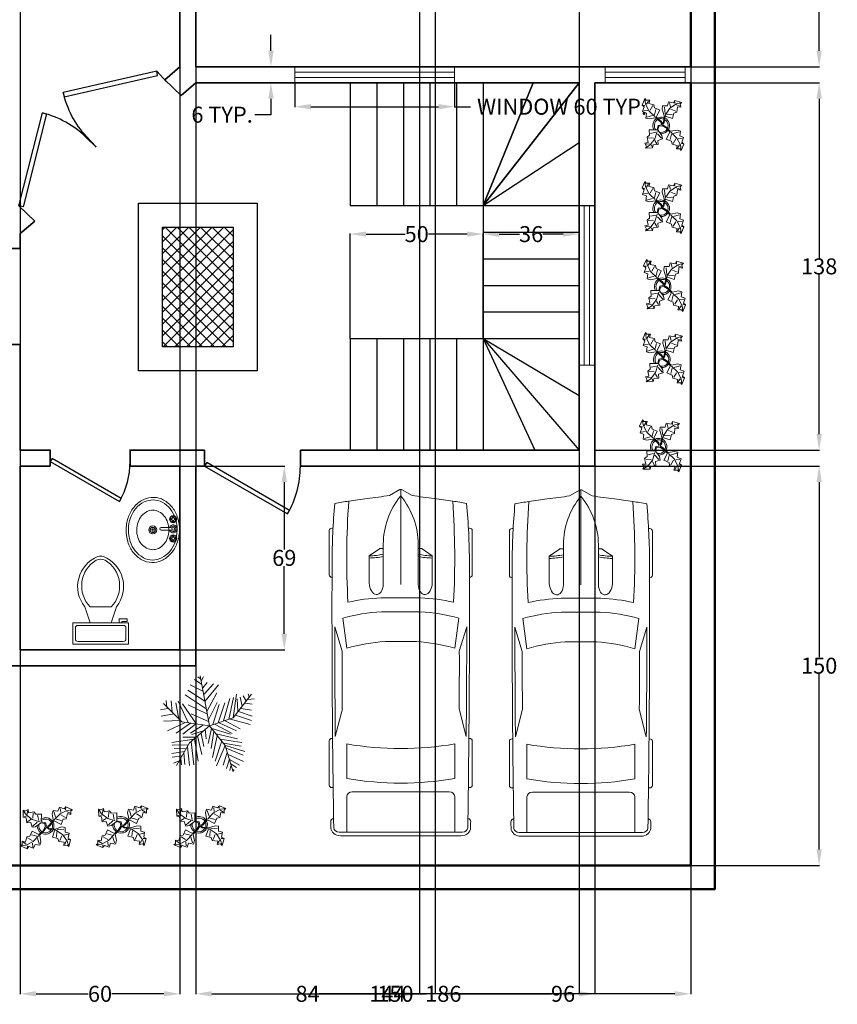
# Model space of a CAD drawing. Units: inches. Extents: x 823 to 1335, y 207 to 1074.
# Tile 2 of 6: x 1028 to 1335, y 207 to 577. Entities that reach past the tile are written whole.
import ezdxf

# ---------------------------------------------------------------- set-up
doc = ezdxf.new("R2010")
doc.units = ezdxf.units.IN
doc.header["$MEASUREMENT"] = 0
for name, color, linetype, lineweight in [('A-ANNO-DIMS', 2, 'Continuous', 18), ('A-EQPM-VEHC', 8, 'Continuous', 13), ('A-FLOR', 7, 'Continuous', 25), ('A-FLOR-PATT', 252, 'Continuous', 13), ('doors', 51, 'Continuous', 25), ('inner wall', 102, 'Continuous', 35), ('L-PLNT', 90, 'Continuous', 13), ('outer wall', 105, 'Continuous', 50), ('sanitary', 131, 'Continuous', 18), ('staircase', 10, 'Continuous', 25), ('windows', 211, 'Continuous', 18)]:
    doc.layers.add(name, color=color, linetype=linetype, lineweight=lineweight)
doc.styles.get("Standard").update_dxf_attribs({"font": 'arial.ttf'})
doc.dimstyles.get("Standard").update_dxf_attribs({"dimtxt": 6, "dimasz": 6, "dimexe": 0.18, "dimexo": 0.0625, "dimgap": 0.09, "dimtad": 0, "dimtih": 1, "dimtoh": 1, "dimdec": 0, "dimzin": 0, "dimdsep": 46, "dimlunit": 3, "dimtxsty": 'Standard', "dimcen": 0.09, "dimadec": 0, "dimazin": 0, "dimtfac": 1, "dimtdec": 0, "dimtofl": 0, "dimtmove": 0, "dimatfit": 3, "dimfxl": 1, "dimtolj": 1, "dimtzin": 0, "dimarcsym": 0})

# ---------------------------------------------------------------- blocks, each defined once
blk = doc.blocks.new('*U5')
for p, q in [((0, 0), (0, -6)), ((-40, 0), (-40, -6))]:
    blk.add_line(p, q)
blk.add_lwpolyline([(0, 0), (-34.64, 20), (-35.52, 18.48), (-0.88, -1.52)], close=True)
blk.add_arc((0, 0), 40, 150, 180)
blk = doc.blocks.new('*U4')
for p, q in [((-40, 0), (-40, 6)), ((0, 0), (0, 6))]:
    blk.add_line(p, q)
blk.add_lwpolyline([(0, 0), (-34.64, -20), (-35.52, -18.48), (-0.88, 1.52)], close=True)
blk.add_arc((0, 0), 40, 180, 210)
blk = doc.blocks.new('*U7')
for p, q in [((0, 0), (0, 6)), ((40, 0), (40, 6))]:
    blk.add_line(p, q)
blk.add_lwpolyline([(0, 0), (34.64, -20), (35.52, -18.48), (0.88, 1.52)], close=True)
blk.add_arc((0, 0), 40, 330, 360)
blk = doc.blocks.new('Toilet - top')
for p, q in [((9.5, -6), (9.5, -2)), ((-10, -8.5), (-8, -8.5)), ((-10, -9.5), (-10, -8.5)), ((-7, -9.5), (-10, -9.5)), ((-8, -8.5), (-8, -8)), ((-7, -8), (-7, -9.5)), ((-4, -8), (-6, -14)), ((4, -8), (6, -14)), ((4, -14), (-4, -14))]:
    blk.add_line(p, q)
blk.add_lwpolyline([(10.5, -8), (10.5, 0), (-10.5, 0), (-10.5, -8)], close=True)
for points in [[(-9.5, -2), (-9.5, -6)], [(8.5, -1), (-8.5, -1)], [(-8.5, -7), (8.5, -7)]]:
    blk.add_lwpolyline(points)
for centre, radius, start, end in [((-8.62, -1.88), 0.884, 81.8699, 188.1301), ((8.62, -1.88), 0.884, 351.8699, 98.1301), ((-8.62, -6.12), 0.884, 171.8699, 278.1301), ((8.62, -6.12), 0.884, 261.8699, 8.1301), ((3.52, -21.58), 12.17, 141.4691, 247.9714), ((4.2, -21.82), 11.33, 136.3677, 238.9468), ((-3.52, -21.58), 12.17, 292.0284, 38.5307), ((-4.2, -21.82), 11.33, 301.053, 43.6321), ((0, -27.88), 4, 245.7318, 294.2682), ((0, -29), 4, 254.8605, 285.1395)]:
    blk.add_arc(centre, radius, start, end)
blk = doc.blocks.new('Sink - Oval top')
for p, q in [((-1, 0), (1, 0)), ((0, 1), (0, -1))]:
    blk.add_line(p, q)
for points in [[(-12.23, 0.39, 0.117634), (-11.46, -3.36, 0.104469), (-8.88, -6.8, 0.090016), (-5.08, -9.07, 0.08192), (-0.32, -10.02, 0.08192), (4.49, -9.38, 0.090016), (8.42, -7.36, 0.104469), (11.22, -4.09, 0.117634), (12.23, -0.39, 0.117634), (11.46, 3.36, 0.104469), (8.88, 6.8, 0.090016), (5.08, 9.07, 0.08192), (0.32, 10.02, 0.08192), (-4.49, 9.38, 0.090016), (-8.42, 7.36, 0.104469), (-11.22, 4.09, 0.117634)], [(-11.29, 0.16, 0.118622), (-10.52, -3.25, 0.104678), (-8.07, -6.36, 0.089562), (-4.54, -8.37, 0.081185), (-0.13, -9.15, 0.081185), (4.3, -8.49, 0.089562), (7.89, -6.58, 0.104678), (10.42, -3.55, 0.118622), (11.29, -0.16, 0.118622), (10.52, 3.25, 0.104678), (8.07, 6.36, 0.089562), (4.54, 8.37, 0.081185), (0.13, 9.15, 0.081185), (-4.3, 8.49, 0.089562), (-7.89, 6.58, 0.104678), (-10.42, 3.55, 0.118622)], [(-7.42, 0.08, 0.118283), (-6.91, -2.17, 0.104607), (-5.29, -4.21, 0.089718), (-2.97, -5.53, 0.081436), (-0.07, -6.04, 0.081436), (2.84, -5.59, 0.089718), (5.2, -4.33, 0.104607), (6.86, -2.32, 0.118283), (7.42, -0.08, 0.118283), (6.91, 2.17, 0.104607), (5.29, 4.21, 0.089718), (2.97, 5.53, 0.081436), (0.07, 6.04, 0.081436), (-2.84, 5.59, 0.089718), (-5.2, 4.33, 0.104607), (-6.86, 2.32, 0.118283)]]:
    blk.add_lwpolyline(points, format="xyb", close=True)
for radius in [1.5, 1]:
    blk.add_circle((0, 0), radius)
blk = doc.blocks.new('Faucet - Bathroom top')
for p, q in [((-4.107, 0.125), (-4.375, 0.125)), ((-3.75, 0.4788), (-3.75, 0.75)), ((-3.5, 0.482), (-3.5, 0.75)), ((-3.1461, 0.125), (-2.875, 0.125)), ((3.143, 0.125), (2.875, 0.125)), ((3.5, 0.4788), (3.5, 0.75)), ((3.75, 0.482), (3.75, 0.75)), ((4.1039, 0.125), (4.375, 0.125)), ((-4.1039, -0.125), (-4.375, -0.125)), ((-3.75, -0.4821), (-3.75, -0.75)), ((-3.5, -0.4789), (-3.5, -0.75)), ((-3.143, -0.125), (-2.875, -0.125)), ((-0.5, -0.8639), (-0.5, -4.5)), ((0.5, -4.5), (0.5, -0.8631)), ((3.1461, -0.125), (2.875, -0.125)), ((3.5, -0.4821), (3.5, -0.75)), ((3.75, -0.4789), (3.75, -0.75)), ((4.107, -0.125), (4.375, -0.125))]:
    blk.add_line(p, q)
for centre, radius in [((-3.625, 0), 1.375), ((-4.625, 0), 0.2795), ((-3.625, 0), 0.5), ((-3.625, 1), 0.2795), ((-2.625, 0), 0.2795), ((0, 0), 0.5), ((3.625, 0), 1.375), ((2.625, 0), 0.2795), ((3.625, 0), 0.5), ((3.625, 1), 0.2795), ((4.625, 0), 0.2795), ((-3.625, -1), 0.2795), ((3.625, -1), 0.2795)]:
    blk.add_circle(centre, radius)
for centre, radius, start, end in [((-3.625, 0), 1, 105.2407, 164.2093), ((-3.625, 0), 1, 16.44125, 74.07887), ((0, 0), 1.5, 289.6514, 250.3603), ((0, 0), 1, 300.3431, 239.7554), ((3.625, 0), 1, 106.12, 164.0884), ((3.625, 0), 1, 16.23422, 73.90469), ((-3.625, 0), 1, 196.2342, 253.9047), ((-3.625, 0), 1, 286.12, 344.0884), ((3.625, 0), 1, 196.4413, 254.0789), ((3.625, 0), 1, 285.2407, 344.2093), ((0, -4.5), 0.5, 180, 0)]:
    blk.add_arc(centre, radius, start, end)
blk = doc.blocks.new('Plant - Rubber or Philodendron')
for p, q in [((-16.2005, 11.4774), (-13.9899, 8.1064)), ((-16.2005, 11.4774), (-14.8639, 10.7964)), ((-16.0159, 6.3329), (-16.2005, 11.4774)), ((-14.8639, 10.7964), (-12.6195, 11.8975)), ((-13.9899, 8.1064), (-9.5434, 4.7185)), ((-13.3174, 8.325), (-13.0735, 11.0065)), ((-12.6195, 11.8975), (-12.1909, 9.4345)), ((-12.1909, 9.4345), (-8.3829, 10.3)), ((-8.8369, 9.409), (-9.0894, 5.6095)), ((-8.3829, 10.3), (-7.0549, 8.501)), ((-7.0549, 8.501), (-3.0284, 8.6941)), ((-4.8529, 4.012), (-5.7184, 7.82)), ((-3.0284, 8.6941), (-3.0709, 3.1041)), ((4.6914, 8.8812), (5.3859, 11.2828)), ((4.6914, 8.8812), (5.5014, 4.4831)), ((5.3859, 11.2828), (8.8871, 10.7908)), ((5.9878, 10.4842), (7.1971, 6.3869)), ((10.3916, 8.7942), (6.2847, 4.4028)), ((8.8871, 10.7908), (9.9809, 13.4933)), ((9.9809, 13.4933), (13.3837, 12.301)), ((15.3859, 11.3055), (10.3916, 8.7942)), ((10.5828, 12.6946), (10.8893, 9.7953)), ((14.2977, 6.1031), (10.9934, 7.9956)), ((13.3837, 12.301), (14.68, 13.9039)), ((14.5816, 13.2037), (14.3848, 11.8033)), ((14.68, 13.9039), (19.3848, 11.8146)), ((15.7909, 9.1065), (14.8995, 5.3044)), ((15.2875, 10.6053), (17.5907, 9.2105)), ((19.3848, 11.8146), (15.3859, 11.3055)), ((18.1925, 8.4119), (15.7909, 9.1065)), ((19.3848, 11.8146), (18.1868, 10.9119)), ((18.1868, 10.9119), (18.1925, 8.4119)), ((-14.0069, 5.8704), (-16.0159, 6.3329)), ((-15.3434, 6.5514), (-13.9984, 6.9884)), ((-13.5868, 2.2894), (-14.0069, 5.8704)), ((-10.6784, 2.491), (-13.5868, 2.2894)), ((-13.1329, 3.1804), (-10.6614, 4.727)), ((-9.5858, -0.8715), (-10.6784, 2.491)), ((-9.5434, 4.7185), (-4.1917, 2.9888)), ((-9.1318, 0.0195), (-5.9793, 2.9025)), ((-7.1228, -0.443), (-3.5248, 2.2131)), ((-3.5248, 2.2131), (-3.3011, 2.4355)), ((-3.3011, 2.4355), (-0.5306, 1.7947)), ((-3.0709, 3.1041), (0.0797, 2.3163)), ((-0.5306, 1.7947), (-0.2255, -0.5527)), ((-0.5306, 1.7947), (-0.5306, 1.7947)), ((0.0797, 2.3163), (0.4866, -0.031)), ((0.4866, -0.031), (2.1141, 0.2298)), ((2.1141, 0.2298), (5.4346, 3.9146)), ((6.1032, 3.6844), (2.8262, -0.031)), ((5.4346, 3.9146), (5.5014, 4.4831)), ((11.1089, 1.1958), (6.1032, 3.6844)), ((7.7005, 4.8881), (11.5025, 3.9967)), ((12.7005, 4.8994), (11.1089, 1.1958)), ((14.8995, 5.3044), (12.7005, 4.8994)), ((-11.3237, -7.2629), (-9.7321, -3.5593)), ((-6.3237, -7.2516), (-10.1257, -6.3602)), ((-9.7321, -3.5593), (-4.7264, -6.0479)), ((-7.1228, -0.443), (-9.5858, -0.8715)), ((-9.0148, -11.1577), (-4.9047, -6.8122)), ((-2.019, -3.6148), (-4.7264, -6.0479)), ((-4.1246, -6.8466), (-4.0579, -6.2781)), ((-3.3146, -11.2447), (-4.1246, -6.8466)), ((-4.0579, -6.2781), (-0.9375, -3.1608)), ((-2.019, -3.6148), (-0.2255, -0.5527)), ((-0.9375, -3.1608), (0.5883, -0.8135)), ((0.5883, -0.8135), (2.2447, -2.0916)), ((2.8262, -0.031), (1.3003, -0.5527)), ((1.3003, -0.5527), (2.4193, -1.4655)), ((2.2447, -2.0916), (6.7108, -2.6626)), ((2.4193, -1.4655), (6.895, -2.1175)), ((4.943, -7.9659), (6.7108, -2.6626)), ((11.6605, -0.5413), (6.895, -2.1175)), ((12.3677, -6.1981), (7.219, -2.6772)), ((8.125, -4.0768), (7.7715, -7.9659)), ((8.3544, -2.7453), (13.1973, -2.1704)), ((10.2463, -10.4408), (11.6605, -6.9053)), ((11.6605, -0.5413), (14.1354, -0.8948)), ((15.5496, -10.7943), (12.3677, -6.1981)), ((16.2567, -5.8446), (13.4283, -6.5517)), ((14.1354, -0.8948), (14.1354, -4.4304)), ((14.1354, -4.4304), (16.9638, -5.1375)), ((16.9638, -5.1375), (16.2567, -8.673)), ((-18.008, -14.1781), (-16.8101, -13.2754)), ((-18.008, -14.1781), (-14.0091, -13.669)), ((-16.8157, -10.7754), (-14.4141, -11.4699)), ((-16.8101, -13.2754), (-16.8157, -10.7754)), ((-13.9107, -12.9688), (-16.2139, -11.574)), ((-14.4141, -11.4699), (-13.5228, -7.6679)), ((-14.0091, -13.669), (-9.0148, -11.1577)), ((-13.5228, -7.6679), (-11.3237, -7.2629)), ((-12.921, -8.4665), (-9.6166, -10.359)), ((-9.206, -15.0581), (-9.5126, -12.1588)), ((-7.5103, -13.1543), (-8.6042, -15.8568)), ((-4.0092, -13.6463), (-7.5103, -13.1543)), ((-4.611, -12.8477), (-5.8203, -8.7504)), ((-3.3146, -11.2447), (-4.0092, -13.6463)), ((8.8321, -9.0266), (4.943, -7.9659)), ((9.5392, -11.1479), (8.8321, -9.0266)), ((13.4283, -11.5015), (9.5392, -11.1479)), ((13.0748, -13.9763), (13.4283, -11.5015)), ((15.5496, -13.6228), (13.0748, -13.9763)), ((14.8425, -10.7943), (13.7819, -13.2692)), ((16.6103, -14.6834), (15.5496, -10.7943)), ((16.6103, -14.6834), (15.5496, -13.6228)), ((17.3174, -9.7337), (15.9032, -9.7337)), ((16.2567, -8.673), (18.0245, -9.7337)), ((18.0245, -9.7337), (16.6103, -14.6834)), ((-13.3032, -16.2674), (-18.008, -14.1781)), ((-12.0069, -14.6645), (-13.3032, -16.2674)), ((-13.2048, -15.5672), (-13.008, -14.1668)), ((-8.6042, -15.8568), (-12.0069, -14.6645))]:
    blk.add_line(p, q)
for centre, radius, start, end in [((0.0308, 0.1664), 6, 178.6147, 235.1169), ((0.0308, 0.1664), 5, 168.1647, 238.6725), ((0, 0), 6.1275, 34.37569, 120.1028), ((-0.0601, -0.2075), 5.2461, 33.82192, 124.9414), ((-0.2664, 0.1682), 5.2775, 338.4094, 20.03007), ((-0.098, 0.1364), 6.1288, 341.2017, 26.09184), ((-0.0234, 0.3825), 6.1492, 242.5812, 331.2714), ((-0.1102, 0.4886), 5.2883, 247.3711, 327.472)]:
    blk.add_arc(centre, radius, start, end)
blk = doc.blocks.new('*U18')
for p, q in [((46.55, 38.89), (22.35, 38.89)), ((136.7, 38.89), (160.9, 38.89)), ((21.1, 37.41), (21.1, 36.83)), ((47.8, 37.39), (47.8, 37.41)), ((87.99, 31.87), (74.76, 35.92)), ((134.31, 35.6), (119.29, 31.78)), ((135.45, 37.07), (135.45, 37.41)), ((162.15, 37.41), (162.15, 36.77)), ((186.47, -33.5), (186.47, 33.5)), ((188.4, -32.76), (188.4, 32.76)), ((70.03, 31.54), (86.41, 29.35)), ((138.42, 29.35), (157.25, 29.35)), ((186.47, 29.35), (167.01, 29.35)), ((164.52, 26.39), (164.52, -26.39)), ((32.27, 11.63), (36.13, 17.17)), ((36.13, 17.17), (50.94, 17.17)), ((32.12, 9.51), (32.12, 11.15)), ((58.92, -10.77), (58.92, 10.77)), ((3.27, 6.13), (0.1, 0.41)), ((29.77, 9.51), (51.68, 9.51)), ((66.55, -10.53), (66.55, 10.53)), ((82.74, 8.5), (82.74, -8.5)), ((186.47, -10.53), (186.47, 10.53)), ((0, 0), (51.68, 0)), ((0.1, -0.41), (3.27, -6.13)), ((29.77, -9.51), (51.68, -9.51)), ((32.12, -9.51), (32.12, -11.15)), ((32.27, -11.63), (36.13, -17.17)), ((36.13, -17.17), (50.94, -17.17)), ((86.41, -29.35), (70.03, -31.54)), ((87.99, -31.87), (74.76, -35.92)), ((134.31, -35.6), (119.29, -31.78)), ((157.25, -29.35), (138.42, -29.35)), ((167.01, -29.35), (186.47, -29.35)), ((21.1, -37.41), (21.1, -36.83)), ((47.8, -37.39), (47.8, -37.41)), ((135.45, -37.07), (135.45, -37.41)), ((162.15, -37.41), (162.15, -36.77)), ((46.55, -38.89), (22.35, -38.89)), ((136.7, -38.89), (160.9, -38.89))]:
    blk.add_line(p, q)
for centre, major_axis, ratio, start_param, end_param in [((22.35, 37.41), (0, -1.48), 0.842304, 3.141593, 4.712389), ((64.48, -10555.62), (0, 10593.03), 0.842304, -0.013397, 0.002797), ((46.55, 37.41), (0, 1.48), 0.842304, -1.570796, 0), ((136.7, 37.41), (0, -1.48), 0.842304, 3.141593, 4.712389), ((160.9, 37.41), (0, 1.48), 0.842304, -1.570796, 0), ((180.63, 35.84), (0, 2.22), 0.842304, -0.013017, 1.249894), ((64.48, -10556.36), (0, 10595.31), 0.842304, -0.013397, -0.013017), ((183.98, 32.76), (0, -5.25), 0.842304, 1.570796, 3.128196), ((266.03, -27.52), (0, 313.31), 0.842304, 1.367076, 1.39176), ((41.19, -490.86), (0, 528.23), 0.842304, 0.00281, 0.075598), ((64.48, -10555.62), (0, -10591.55), 0.842304, 3.133765, 3.140441), ((183.98, 33.5), (0, -2.96), 0.842304, 1.570796, 3.128196), ((259.18, -27.52), (0, -305.3), 0.842304, 4.528606, 4.561838), ((37.47, -593.96), (0, -623.33), 0.842304, 3.096046, 3.200911), ((134.4, 5.39), (0, -89.78), 0.842304, 4.449482, 4.652344), ((135.29, 5.39), (0, 81.77), 0.842304, 1.245306, 1.50788), ((149.6, 2.8), (0, -79.58), 0.842304, 4.372215, 4.640744), ((95.79, -3666.35), (0, -3698.24), 0.842304, 3.134049, 3.144098), ((17.08, 0), (0, 147.02), 0.842304, 4.511394, 4.913384), ((35.91, 0), (0, 147.02), 0.842304, 4.511394, 4.913384), ((167.01, 26.39), (0, 2.96), 0.842304, 0, 1.570796), ((-204.49, 52.4), (0, -250.96), 0.842304, 1.385369, 1.434372), ((13.04, 17.01), (0, 27.42), 0.842304, 4.435146, 4.718221), ((14.2, 17.01), (0, 27.42), 0.842304, 4.435146, 4.718221), ((50.79, 13.34), (6.34, -0.36), 0.603834, -1.395552, 1.581315), ((32.75, 11.15), (0, 0.74), 0.842304, 0.879714, 1.570796), ((29.77, -46.66), (0, 56.17), 0.842304, 0, 0.590319), ((0.62, 0), (0, -0.74), 0.842304, 4.131459, 5.293319), ((29.77, 46.66), (0, 56.17), 0.842304, 2.551274, 3.141593), ((-204.49, -52.4), (0, 250.96), 0.842304, -1.434372, -1.385369), ((13.04, -17.01), (0, -27.42), 0.842304, 1.564964, 1.848039), ((14.2, -17.01), (0, -27.42), 0.842304, 1.564964, 1.848039), ((135.29, -5.39), (0, -81.77), 0.842304, -1.50788, -1.245306), ((149.6, -2.8), (0, -79.58), 0.842304, -1.499151, -1.230623), ((32.75, -11.15), (0, -0.74), 0.842304, 4.712389, 5.403472), ((134.4, -5.39), (0, -89.78), 0.842304, -1.510751, -1.307889), ((259.18, 27.52), (0, 305.3), 0.842304, 1.721348, 1.754579), ((167.01, -26.39), (0, -2.96), 0.842304, 4.712389, 6.283185), ((266.03, 27.52), (0, 313.31), 0.842304, 1.749832, 1.774517), ((37.47, 593.96), (0, -623.33), 0.842304, -0.059319, 0.045547), ((95.79, 3666.35), (0, -3698.24), 0.842304, -0.002505, 0.007544), ((41.19, 490.86), (0, -528.23), 0.842304, -0.075598, -0.00281), ((22.35, -37.41), (0, 1.48), 0.842304, 1.570796, 3.141593), ((64.48, 10555.62), (0, 10593.03), 0.842304, 3.138796, 3.15499), ((46.55, -37.41), (0, -1.48), 0.842304, 0, 1.570796), ((64.48, 10555.62), (0, -10591.55), 0.842304, 0.001152, 0.007828), ((136.7, -37.41), (0, -1.48), 0.842304, -1.570796, 0), ((160.9, -37.41), (0, 1.48), 0.842304, 3.141593, 4.712389), ((180.63, -35.84), (0, -2.22), 0.842304, -1.249894, 0.013017), ((183.98, -33.5), (0, 2.96), 0.842304, 3.15499, 4.712389), ((183.98, -32.76), (0, -5.25), 0.842304, 0.013397, 1.570796), ((64.48, 10556.36), (0, 10595.31), 0.842304, 3.15461, 3.15499)]:
    blk.add_ellipse(centre, major_axis=major_axis, ratio=ratio, start_param=start_param, end_param=end_param)
at = {"extrusion": (0, 0, -1)}
blk.add_ellipse((50.79, -13.34), major_axis=(6.34, 0.36), ratio=0.603834, start_param=-1.395552, end_param=1.581315, dxfattribs=at)
blk = doc.blocks.new('*U20')
for p, q in [((0, 0), (-10.5, 57)), ((-7.288, 39.707), (-21.778, 46.673)), ((-8.737, 47.138), (-17.069, 52.711)), ((-10.186, 53.64), (-13.084, 55.962)), ((-9.099, 51.782), (-6.563, 55.962)), ((-7.65, 43.423), (-2.578, 49.46)), ((-5.839, 35.992), (4.667, 48.067)), ((-5.114, 27.632), (10.463, 46.673)), ((-3.665, 19.273), (-27.574, 35.527)), ((-5.114, 28.097), (-24.676, 40.636)), ((-2.941, 16.486), (8.652, 37.85)), ((27, 9), (48, 36)), ((27.127, 9.056), (31.112, 35.992)), ((38.719, 34.134), (41.979, 28.561)), ((44.153, 36.456), (45.239, 32.741)), ((-31.5, 4.5), (-52.5, 25.5)), ((-48.585, 21.131), (-49.309, 29.026)), ((-43.513, 28.561), (-42.427, 15.558)), ((-38.442, 26.239), (-34.819, 7.663)), ((-35.544, 28.097), (-24.314, 3.947)), ((-14.533, 2.09), (-30.834, 25.31)), ((-24.314, 23.917), (-2.941, 13.7)), ((-1.129, 6.734), (9.014, 26.704)), ((3.942, 1.625), (11.187, 24.381)), ((10.101, 3.483), (17.708, 26.239)), ((16.259, 5.805), (23.142, 31.348)), ((22.055, 7.198), (27.489, 32.277)), ((31.836, 30.883), (32.561, 16.486)), ((35.096, 32.741), (37.27, 22.524)), ((40.53, 25.775), (48.862, 24.846)), ((43.791, 29.954), (51.036, 30.883)), ((-47.498, 19.737), (-55.83, 18.344)), ((-40.615, 13.7), (-55.105, 10.913)), ((-20.691, 13.7), (-1.129, 4.876)), ((29.662, 12.307), (48.137, 6.269)), ((33.285, 16.486), (48.862, 10.913)), ((36.183, 19.737), (48.137, 17.88)), ((-33.37, 6.269), (-52.207, 5.34)), ((-28.299, 3.483), (-47.86, -5.805)), ((-21.416, 3.018), (-38.079, -8.128)), ((0, 0), (-31.5, 4.5)), ((-15.982, 2.09), (-30.11, -9.521)), ((0, 0), (-22.5, -19.5)), ((-6.563, 1.161), (-21.416, -8.128)), ((0, 0), (27, 9)), ((0, 0), (18, -22.5)), ((6.478, 1.625), (26.04, -8.592)), ((11.187, 3.483), (30.749, -5.805)), ((18.07, 5.805), (35.096, -3.483)), ((24.229, 7.663), (46.688, 1.625)), ((-6.563, -5.805), (-19.967, -9.985)), ((-9.461, -8.592), (-6.201, -23.453)), ((-4.752, -3.483), (-3.665, -14.629)), ((2.493, -3.019), (-1.491, -20.202)), ((1.769, -2.555), (24.229, -9.521)), ((5.029, -6.27), (2.131, -25.775)), ((7.565, -9.056), (32.198, -14.629)), ((-17.431, -15.094), (-42.789, -18.809)), ((-24.314, -21.596), (-42.427, -22.06)), ((-22.5, -19.5), (-37.5, -45)), ((-15.257, -12.772), (-30.11, -12.772)), ((-20.691, -18.345), (-17.793, -44.352)), ((-17.069, -15.094), (-12.721, -40.172)), ((-13.446, -11.378), (-8.737, -32.741)), ((9.014, -11.378), (3.58, -35.992)), ((14.085, -16.951), (6.478, -40.172)), ((12.274, -15.094), (36.907, -18.809)), ((16.259, -19.738), (36.183, -22.989)), ((-28.299, -29.026), (-42.789, -31.348)), ((-26.849, -26.24), (-40.253, -25.775)), ((-29.023, -30.884), (-27.936, -43.887)), ((-25.038, -23.918), (-22.865, -45.281)), ((18.07, -22.524), (8.289, -45.745)), ((20.244, -30.419), (15.897, -44.816)), ((18, -22.5), (27, -52.5)), ((18.433, -22.524), (40.53, -29.026)), ((19.157, -25.311), (38.719, -33.206)), ((21.331, -32.741), (39.081, -40.636)), ((-30.834, -34.135), (-42.427, -35.528)), ((-34.457, -39.708), (-40.978, -42.494)), ((-32.646, -36.921), (-31.921, -44.352)), ((22.78, -37.85), (19.519, -48.532)), ((22.78, -38.314), (34.372, -44.816)), ((24.591, -43.423), (30.749, -47.603)), ((24.591, -45.745), (23.142, -50.854)), ((26.764, -49.925), (28.213, -50.854))]:
    blk.add_line(p, q)
blk = doc.blocks.new('WIN-60IN')
for p, q in [((0, 0), (0, 60)), ((0, 60), (6, 60)), ((2, 0), (2, 60)), ((4, 60), (4, 0)), ((6, 60), (6, 0)), ((6, 0), (0, 0))]:
    blk.add_line(p, q)
blk = doc.blocks.new('WIN-30IN')
for p, q in [((0, 6), (30, 6)), ((0, 0), (0, 6)), ((0, 4), (30, 4)), ((30, 6), (30, 0)), ((30, 2), (0, 2)), ((30, 0), (0, 0))]:
    blk.add_line(p, q)
blk = doc.blocks.new('*D46')
at = {"layer": 'A-ANNO-DIMS', "color": 0, "lineweight": -2, "transparency": 16777216}
for p, q in [((1131.5, 553.54), (1131.5, 544.43)), ((1191.5, 553.54), (1191.5, 544.43)), ((1137.5, 544.61), (1185.5, 544.61)), ((1191.5, 544.61), (1197.5, 544.61))]:
    blk.add_line(p, q, dxfattribs=at)
for points in [[(1137.5, 545.61), (1137.5, 543.61), (1131.5, 544.61)], [(1185.5, 545.61), (1185.5, 543.61), (1191.5, 544.61)]]:
    blk.add_solid(points, dxfattribs=at)
at = {"layer": 'Defpoints', "color": 0, "lineweight": -2, "transparency": 16777216}
for p in [(1131.5, 553.61), (1191.5, 553.61), (1191.5, 544.61)]:
    blk.add_point(p, dxfattribs=at)
at = {"layer": 'A-ANNO-DIMS', "color": 0, "transparency": 16777216, "insert": (1231.87, 544.61), "char_height": 6, "attachment_point": 5}
blk.add_mtext('\\A1;WINDOW 60 TYP.', dxfattribs=at)
blk = doc.blocks.new('*D47')
at = {"layer": 'A-ANNO-DIMS', "color": 0, "lineweight": -2, "transparency": 16777216}
for p, q in [((1122.5, 565.61), (1122.5, 571.61)), ((1131.44, 559.61), (1122.32, 559.61)), ((1131.44, 553.61), (1122.32, 553.61)), ((1122.5, 547.61), (1122.5, 541.61)), ((1122.5, 541.61), (1116.5, 541.61))]:
    blk.add_line(p, q, dxfattribs=at)
for points in [[(1121.5, 565.61), (1123.5, 565.61), (1122.5, 559.61)], [(1121.5, 547.61), (1123.5, 547.61), (1122.5, 553.61)]]:
    blk.add_solid(points, dxfattribs=at)
at = {"layer": 'Defpoints', "color": 0, "lineweight": -2, "transparency": 16777216}
for p in [(1131.5, 559.61), (1122.5, 553.61), (1131.5, 553.61)]:
    blk.add_point(p, dxfattribs=at)
at = {"layer": 'A-ANNO-DIMS', "color": 0, "transparency": 16777216, "insert": (1104.13, 541.61), "char_height": 6, "attachment_point": 5}
blk.add_mtext('\\A1;6 TYP.', dxfattribs=at)
blk = doc.blocks.new('*D61')
at = {"layer": 'A-ANNO-DIMS', "color": 0, "lineweight": -2, "transparency": 16777216}
for p, q in [((1028.26, 847.54), (1028.26, 211.18)), ((1088.26, 847.54), (1088.26, 211.18)), ((1034.26, 211.36), (1053.87, 211.36)), ((1082.26, 211.36), (1062.66, 211.36))]:
    blk.add_line(p, q, dxfattribs=at)
for points in [[(1034.26, 212.36), (1034.26, 210.36), (1028.26, 211.36)], [(1082.26, 212.36), (1082.26, 210.36), (1088.26, 211.36)]]:
    blk.add_solid(points, dxfattribs=at)
at = {"layer": 'Defpoints', "color": 0, "lineweight": -2, "transparency": 16777216}
for p in [(1028.26, 847.61), (1088.26, 847.61), (1088.26, 211.36)]:
    blk.add_point(p, dxfattribs=at)
at = {"layer": 'A-ANNO-DIMS', "color": 0, "transparency": 16777216, "insert": (1058.26, 211.36), "char_height": 6, "attachment_point": 5}
blk.add_mtext('\\A1;60', dxfattribs=at)
blk = doc.blocks.new('*D62')
at = {"layer": 'A-ANNO-DIMS', "color": 0, "lineweight": -2, "transparency": 16777216}
for p, q in [((1094.26, 775.54), (1094.26, 211.18)), ((1238.26, 775.54), (1238.26, 211.18)), ((1100.26, 211.36), (1159.84, 211.36)), ((1232.26, 211.36), (1172.69, 211.36))]:
    blk.add_line(p, q, dxfattribs=at)
for points in [[(1100.26, 212.36), (1100.26, 210.36), (1094.26, 211.36)], [(1232.26, 212.36), (1232.26, 210.36), (1238.26, 211.36)]]:
    blk.add_solid(points, dxfattribs=at)
at = {"layer": 'Defpoints', "color": 0, "lineweight": -2, "transparency": 16777216}
for p in [(1094.26, 775.61), (1238.26, 775.61), (1238.26, 211.36)]:
    blk.add_point(p, dxfattribs=at)
at = {"layer": 'A-ANNO-DIMS', "color": 0, "transparency": 16777216, "insert": (1166.26, 211.36), "char_height": 6, "attachment_point": 5}
blk.add_mtext('\\A1;144', dxfattribs=at)
blk = doc.blocks.new('*D68')
at = {"layer": 'A-ANNO-DIMS', "color": 0, "lineweight": -2, "transparency": 16777216}
for p, q in [((1094.26, 709.54), (1094.26, 211.18)), ((1178.26, 709.54), (1178.26, 211.18)), ((1100.26, 211.36), (1131.88, 211.36)), ((1172.26, 211.36), (1140.64, 211.36))]:
    blk.add_line(p, q, dxfattribs=at)
for points in [[(1100.26, 212.36), (1100.26, 210.36), (1094.26, 211.36)], [(1172.26, 212.36), (1172.26, 210.36), (1178.26, 211.36)]]:
    blk.add_solid(points, dxfattribs=at)
at = {"layer": 'Defpoints', "color": 0, "lineweight": -2, "transparency": 16777216}
for p in [(1094.26, 709.61), (1178.26, 709.61), (1178.26, 211.36)]:
    blk.add_point(p, dxfattribs=at)
at = {"layer": 'A-ANNO-DIMS', "color": 0, "transparency": 16777216, "insert": (1136.26, 211.36), "char_height": 6, "attachment_point": 5}
blk.add_mtext('\\A1;84', dxfattribs=at)
blk = doc.blocks.new('*D69')
at = {"layer": 'A-ANNO-DIMS', "color": 0, "lineweight": -2, "transparency": 16777216}
for p, q in [((1184.26, 709.54), (1184.26, 211.18)), ((1280.26, 709.54), (1280.26, 211.18)), ((1190.26, 211.36), (1227.88, 211.36)), ((1274.26, 211.36), (1236.65, 211.36))]:
    blk.add_line(p, q, dxfattribs=at)
for points in [[(1190.26, 212.36), (1190.26, 210.36), (1184.26, 211.36)], [(1274.26, 212.36), (1274.26, 210.36), (1280.26, 211.36)]]:
    blk.add_solid(points, dxfattribs=at)
at = {"layer": 'Defpoints', "color": 0, "lineweight": -2, "transparency": 16777216}
for p in [(1184.26, 709.61), (1280.26, 709.61), (1280.26, 211.36)]:
    blk.add_point(p, dxfattribs=at)
at = {"layer": 'A-ANNO-DIMS', "color": 0, "transparency": 16777216, "insert": (1232.26, 211.36), "char_height": 6, "attachment_point": 5}
blk.add_mtext('\\A1;96', dxfattribs=at)
blk = doc.blocks.new('*D71')
at = {"layer": 'A-ANNO-DIMS', "color": 0, "lineweight": -2, "transparency": 16777216}
for p, q in [((1094.26, 559.54), (1094.26, 211.18)), ((1280.26, 559.54), (1280.26, 211.18)), ((1100.26, 211.36), (1180.83, 211.36)), ((1274.26, 211.36), (1193.7, 211.36))]:
    blk.add_line(p, q, dxfattribs=at)
for points in [[(1100.26, 212.36), (1100.26, 210.36), (1094.26, 211.36)], [(1274.26, 212.36), (1274.26, 210.36), (1280.26, 211.36)]]:
    blk.add_solid(points, dxfattribs=at)
at = {"layer": 'Defpoints', "color": 0, "lineweight": -2, "transparency": 16777216}
for p in [(1094.26, 559.61), (1280.26, 559.61), (1280.26, 211.36)]:
    blk.add_point(p, dxfattribs=at)
at = {"layer": 'A-ANNO-DIMS', "color": 0, "transparency": 16777216, "insert": (1187.26, 211.36), "char_height": 6, "attachment_point": 5}
blk.add_mtext('\\A1;186', dxfattribs=at)
blk = doc.blocks.new('*D72')
at = {"layer": 'A-ANNO-DIMS', "color": 0, "lineweight": -2, "transparency": 16777216}
for p, q in [((1280.32, 703.61), (1328.69, 703.61)), ((1328.51, 697.61), (1328.51, 634.71)), ((1328.51, 565.61), (1328.51, 628.5)), ((1280.32, 559.61), (1328.69, 559.61))]:
    blk.add_line(p, q, dxfattribs=at)
for points in [[(1327.51, 697.61), (1329.51, 697.61), (1328.51, 703.61)], [(1327.51, 565.61), (1329.51, 565.61), (1328.51, 559.61)]]:
    blk.add_solid(points, dxfattribs=at)
at = {"layer": 'Defpoints', "color": 0, "lineweight": -2, "transparency": 16777216}
for p in [(1280.26, 703.61), (1328.51, 703.61), (1280.26, 559.61)]:
    blk.add_point(p, dxfattribs=at)
at = {"layer": 'A-ANNO-DIMS', "color": 0, "transparency": 16777216, "insert": (1328.51, 631.61), "char_height": 6, "attachment_point": 5}
blk.add_mtext('\\A1;144', dxfattribs=at)
blk = doc.blocks.new('*D75')
at = {"layer": 'A-ANNO-DIMS', "color": 0, "lineweight": -2, "transparency": 16777216}
for p, q in [((1028.26, 340.54), (1028.26, 211.18)), ((1088.26, 340.54), (1088.26, 211.18)), ((1034.26, 211.36), (1053.87, 211.36)), ((1082.26, 211.36), (1062.66, 211.36))]:
    blk.add_line(p, q, dxfattribs=at)
for points in [[(1034.26, 212.36), (1034.26, 210.36), (1028.26, 211.36)], [(1082.26, 212.36), (1082.26, 210.36), (1088.26, 211.36)]]:
    blk.add_solid(points, dxfattribs=at)
at = {"layer": 'Defpoints', "color": 0, "lineweight": -2, "transparency": 16777216}
for p in [(1028.26, 340.61), (1088.26, 340.61), (1088.26, 211.36)]:
    blk.add_point(p, dxfattribs=at)
at = {"layer": 'A-ANNO-DIMS', "color": 0, "transparency": 16777216, "insert": (1058.26, 211.36), "char_height": 6, "attachment_point": 5}
blk.add_mtext('\\A1;60', dxfattribs=at)
blk = doc.blocks.new('*D76')
at = {"layer": 'A-ANNO-DIMS', "color": 0, "lineweight": -2, "transparency": 16777216}
for p, q in [((1088.32, 409.61), (1127.69, 409.61)), ((1127.51, 403.61), (1127.51, 378.26)), ((1127.51, 346.61), (1127.51, 371.95)), ((1088.32, 340.61), (1127.69, 340.61))]:
    blk.add_line(p, q, dxfattribs=at)
for points in [[(1126.51, 403.61), (1128.51, 403.61), (1127.51, 409.61)], [(1126.51, 346.61), (1128.51, 346.61), (1127.51, 340.61)]]:
    blk.add_solid(points, dxfattribs=at)
at = {"layer": 'Defpoints', "color": 0, "lineweight": -2, "transparency": 16777216}
for p in [(1088.26, 409.61), (1088.26, 340.61), (1127.51, 340.61)]:
    blk.add_point(p, dxfattribs=at)
at = {"layer": 'A-ANNO-DIMS', "color": 0, "transparency": 16777216, "insert": (1127.51, 375.11), "char_height": 6, "attachment_point": 5}
blk.add_mtext('\\A1;69', dxfattribs=at)
blk = doc.blocks.new('*D77')
at = {"layer": 'A-ANNO-DIMS', "color": 0, "lineweight": -2, "transparency": 16777216}
for p, q in [((1094.26, 409.54), (1094.26, 211.18)), ((1244.26, 409.54), (1244.26, 211.18)), ((1100.26, 211.36), (1162.84, 211.36)), ((1238.26, 211.36), (1175.69, 211.36))]:
    blk.add_line(p, q, dxfattribs=at)
for points in [[(1100.26, 212.36), (1100.26, 210.36), (1094.26, 211.36)], [(1238.26, 212.36), (1238.26, 210.36), (1244.26, 211.36)]]:
    blk.add_solid(points, dxfattribs=at)
at = {"layer": 'Defpoints', "color": 0, "lineweight": -2, "transparency": 16777216}
for p in [(1094.26, 409.61), (1244.26, 409.61), (1244.26, 211.36)]:
    blk.add_point(p, dxfattribs=at)
at = {"layer": 'A-ANNO-DIMS', "color": 0, "transparency": 16777216, "insert": (1169.26, 211.36), "char_height": 6, "attachment_point": 5}
blk.add_mtext('\\A1;150', dxfattribs=at)
blk = doc.blocks.new('*D78')
at = {"layer": 'A-ANNO-DIMS', "color": 0, "lineweight": -2, "transparency": 16777216}
for p, q in [((1244.32, 553.61), (1328.69, 553.61)), ((1328.51, 547.61), (1328.51, 487.76)), ((1328.51, 421.61), (1328.51, 481.45)), ((1244.32, 415.61), (1328.69, 415.61))]:
    blk.add_line(p, q, dxfattribs=at)
for points in [[(1327.51, 547.61), (1329.51, 547.61), (1328.51, 553.61)], [(1327.51, 421.61), (1329.51, 421.61), (1328.51, 415.61)]]:
    blk.add_solid(points, dxfattribs=at)
at = {"layer": 'Defpoints', "color": 0, "lineweight": -2, "transparency": 16777216}
for p in [(1244.26, 553.61), (1328.51, 553.61), (1244.26, 415.61)]:
    blk.add_point(p, dxfattribs=at)
at = {"layer": 'A-ANNO-DIMS', "color": 0, "transparency": 16777216, "insert": (1328.51, 484.61), "char_height": 6, "attachment_point": 5}
blk.add_mtext('\\A1;138', dxfattribs=at)
blk = doc.blocks.new('*D79')
at = {"layer": 'A-ANNO-DIMS', "color": 0, "lineweight": -2, "transparency": 16777216}
for p, q in [((1244.32, 409.61), (1328.69, 409.61)), ((1328.51, 403.61), (1328.51, 337.76)), ((1328.51, 265.61), (1328.51, 331.45)), ((1280.32, 259.61), (1328.69, 259.61))]:
    blk.add_line(p, q, dxfattribs=at)
for points in [[(1327.51, 403.61), (1329.51, 403.61), (1328.51, 409.61)], [(1327.51, 265.61), (1329.51, 265.61), (1328.51, 259.61)]]:
    blk.add_solid(points, dxfattribs=at)
at = {"layer": 'Defpoints', "color": 0, "lineweight": -2, "transparency": 16777216}
for p in [(1244.26, 409.61), (1328.51, 409.61), (1280.26, 259.61)]:
    blk.add_point(p, dxfattribs=at)
at = {"layer": 'A-ANNO-DIMS', "color": 0, "transparency": 16777216, "insert": (1328.51, 334.61), "char_height": 6, "attachment_point": 5}
blk.add_mtext('\\A1;150', dxfattribs=at)
blk = doc.blocks.new('*D80')
at = {"layer": 'A-ANNO-DIMS', "color": 0, "lineweight": -2, "transparency": 16777216}
for p, q in [((1152.26, 457.56), (1152.26, 496.93)), ((1158.26, 496.75), (1172.88, 496.75)), ((1196.26, 496.75), (1181.64, 496.75)), ((1202.26, 457.56), (1202.26, 496.93))]:
    blk.add_line(p, q, dxfattribs=at)
for points in [[(1158.26, 497.75), (1158.26, 495.75), (1152.26, 496.75)], [(1196.26, 497.75), (1196.26, 495.75), (1202.26, 496.75)]]:
    blk.add_solid(points, dxfattribs=at)
at = {"layer": 'Defpoints', "color": 0, "lineweight": -2, "transparency": 16777216}
for p in [(1202.26, 496.75), (1152.26, 457.5), (1202.26, 457.5)]:
    blk.add_point(p, dxfattribs=at)
at = {"layer": 'A-ANNO-DIMS', "color": 0, "transparency": 16777216, "insert": (1177.26, 496.75), "char_height": 6, "attachment_point": 5}
blk.add_mtext('\\A1;50', dxfattribs=at)
blk = doc.blocks.new('*D81')
at = {"layer": 'A-ANNO-DIMS', "color": 0, "lineweight": -2, "transparency": 16777216}
for p, q in [((1202.26, 457.56), (1202.26, 496.93)), ((1208.26, 496.75), (1215.88, 496.75)), ((1232.26, 496.75), (1224.65, 496.75)), ((1238.26, 457.56), (1238.26, 496.93))]:
    blk.add_line(p, q, dxfattribs=at)
for points in [[(1208.26, 497.75), (1208.26, 495.75), (1202.26, 496.75)], [(1232.26, 497.75), (1232.26, 495.75), (1238.26, 496.75)]]:
    blk.add_solid(points, dxfattribs=at)
at = {"layer": 'Defpoints', "color": 0, "lineweight": -2, "transparency": 16777216}
for p in [(1238.26, 496.75), (1202.26, 457.5), (1238.26, 457.5)]:
    blk.add_point(p, dxfattribs=at)
at = {"layer": 'A-ANNO-DIMS', "color": 0, "transparency": 16777216, "insert": (1220.26, 496.75), "char_height": 6, "attachment_point": 5}
blk.add_mtext('\\A1;36', dxfattribs=at)

msp = doc.modelspace()

# ---------------------------------------------------------------- hatches: boundary and pattern name
at = {"layer": 'A-FLOR-PATT'}
h = msp.add_hatch(dxfattribs=at)
h.set_pattern_fill('ANSI37', color=256, scale=25)
h.paths.add_polyline_path([(1108.26, 499.38), (1081.68, 499.38), (1081.68, 454.4), (1108.26, 454.4)])

# ---------------------------------------------------------------- linework, layer by layer
at = {"layer": 'A-FLOR'}
for points in [[(1072.68, 508.38), (1117.26, 508.38), (1117.26, 445.4), (1072.68, 445.4)], [(1081.68, 499.38), (1108.26, 499.38), (1108.26, 454.4), (1081.68, 454.4)]]:
    msp.add_lwpolyline(points, close=True, dxfattribs=at)
at = {"layer": 'inner wall'}
for p, q in [((1088.26, 663.21), (1088.26, 559.61)), ((1094.26, 663.21), (1094.26, 559.61)), ((1082.61, 554.72), (1088.26, 559.61)), ((1094.26, 559.61), (1280.26, 559.61)), ((1082.62, 554.73), (1088.7, 548.83)), ((1088.7, 548.83), (1094.26, 553.61)), ((1094.26, 553.61), (1238.26, 553.61)), ((1238.26, 553.61), (1238.26, 415.61)), ((1244.26, 553.61), (1244.26, 415.61)), ((1244.26, 553.61), (1280.26, 553.61)), ((1027.79, 507.38), (1033.71, 501.63)), ((1028.26, 496.95), (1033.71, 501.63)), ((1028.26, 491.3), (1028.26, 496.95)), ((1028.26, 415.61), (1028.26, 455.3)), ((1039.56, 415.61), (1028.26, 415.61)), ((1088.26, 415.61), (1069.56, 415.61)), ((1088.26, 415.61), (1097.55, 415.61)), ((1088.26, 415.61), (1097.55, 415.61)), ((1133.55, 415.61), (1238.26, 415.61)), ((1133.55, 415.61), (1238.26, 415.61)), ((1244.26, 415.61), (1244.26, 409.61)), ((1028.26, 340.61), (1028.26, 409.61)), ((1039.56, 409.61), (1028.26, 409.61)), ((1088.26, 409.61), (1069.56, 409.61)), ((1088.26, 409.61), (1088.26, 340.61)), ((1088.26, 409.61), (1088.26, 340.61)), ((1094.26, 409.61), (1097.55, 409.61)), ((1094.26, 409.61), (1094.26, 334.61)), ((1133.55, 409.61), (1244.26, 409.61)), ((1088.26, 340.61), (1028.26, 340.61)), ((1088.26, 334.61), (878.26, 334.61)), ((1088.26, 334.61), (1094.26, 334.61))]:
    msp.add_line(p, q, dxfattribs=at)
for points in [[(1028.26, 491.3), (1022.26, 491.3)], [(1022.26, 455.3), (1028.26, 455.3)], [(1039.56, 409.61), (1039.56, 415.61)], [(1069.56, 415.61), (1069.56, 409.61)], [(1097.55, 415.61), (1097.55, 409.61)], [(1133.55, 409.61), (1133.55, 415.61)]]:
    msp.add_lwpolyline(points, dxfattribs=at)
at = {"layer": 'outer wall'}
for p, q in [((1280.26, 703.61), (1280.26, 559.61)), ((1280.26, 553.61), (1280.26, 259.61)), ((1280.26, 259.61), (878.26, 259.61))]:
    msp.add_line(p, q, dxfattribs=at)
msp.add_lwpolyline([(869.26, 1030.61), (1289.26, 1030.61), (1289.26, 250.61), (869.26, 250.61)], close=True, dxfattribs=at)
at = {"layer": 'staircase'}
for p, q in [((1152.26, 553.61), (1152.26, 507.5)), ((1162.26, 553.61), (1162.26, 507.5)), ((1172.26, 553.61), (1172.26, 507.5)), ((1182.26, 553.61), (1182.26, 507.5)), ((1192.26, 553.61), (1192.26, 507.5)), ((1202.26, 553.61), (1202.26, 415.61)), ((1202.26, 507.5), (1221.02, 553.61)), ((1221.02, 553.61), (1202.26, 507.5)), ((1202.26, 507.5), (1238.26, 553.61)), ((1238.26, 553.61), (1202.26, 507.5)), ((1202.26, 507.5), (1238.26, 531.15)), ((1152.26, 507.5), (1244.26, 507.5)), ((1202.26, 497.5), (1238.26, 497.5)), ((1202.26, 487.5), (1238.26, 487.5)), ((1202.26, 477.5), (1238.26, 477.5)), ((1202.26, 467.5), (1238.26, 467.5)), ((1152.26, 457.5), (1238.26, 457.5)), ((1152.26, 457.5), (1152.26, 415.61)), ((1162.26, 457.5), (1162.26, 415.61)), ((1172.26, 457.5), (1172.26, 415.61)), ((1182.26, 457.5), (1182.26, 415.61)), ((1192.26, 457.5), (1192.26, 415.61)), ((1202.26, 457.5), (1238.26, 415.61)), ((1202.26, 457.5), (1221.61, 415.61)), ((1202.26, 457.5), (1238.26, 436.15))]:
    msp.add_line(p, q, dxfattribs=at)

# ---------------------------------------------------------------- block references
at = {"layer": 'A-EQPM-VEHC', "xscale": 0.6906349484842726, "yscale": 0.6906349484842726, "zscale": 0.6906349484842726, "rotation": 270}
for p in [(1171.27, 400.83), (1238.96, 400.69)]:
    msp.add_blockref('*U18', p, dxfattribs=at)
at = {"layer": 'doors'}
for name, p, xscale, yscale, zscale, rotation in [('*U4', (1079.56, 557.91), -0.9000000000000001, 0.9000000000000001, 0.9000000000000001, 222.8493564413875), ('*U4', (1027.79, 507.38), 0.9000000000000001, 0.9000000000000001, 0.9000000000000001, 225.7621076971286), ('*U5', (1022.86, 491.3), 0.9, 0.9, 0.9, 90), ('*U5', (1039.56, 411.27), 0.75, 0.75, 0.75, 180)]:
    msp.add_blockref(name, p, dxfattribs=dict(at, xscale=xscale, yscale=yscale, zscale=zscale, rotation=rotation))
at = {"layer": 'doors', "xscale": 0.9, "yscale": 0.9, "zscale": 0.9}
msp.add_blockref('*U7', (1097.55, 409.61), dxfattribs=at)
at = {"layer": 'L-PLNT', "xscale": 0.5226467583176748, "yscale": 0.5226467583176748, "zscale": 0.5226467583176748, "rotation": 90}
for p in [(1269.21, 537.54), (1269.21, 506.42), (1269.82, 477.13), (1269.46, 449.7), (1268.3, 416.87)]:
    msp.add_blockref('Plant - Rubber or Philodendron', p, dxfattribs=at)
at = {"layer": 'L-PLNT'}
for name, p, xscale, yscale, zscale in [('*U20', (1099.36, 312.01), 0.3294393859005505, 0.3294393859005505, 0.3294393859005505), ('Plant - Rubber or Philodendron', (1037.8, 274.36), 0.5226467583176748, 0.5226467583176748, 0.5226467583176748), ('Plant - Rubber or Philodendron', (1066.17, 274.77), 0.5226467583176748, 0.5226467583176748, 0.5226467583176748), ('Plant - Rubber or Philodendron', (1095.46, 274.77), 0.5226467583176748, 0.5226467583176748, 0.5226467583176748)]:
    msp.add_blockref(name, p, dxfattribs=dict(at, xscale=xscale, yscale=yscale, zscale=zscale))
at = {"layer": 'sanitary'}
for name, p, rotation in [('Sink - Oval top', (1078.09, 385.61), 89.99999999999999), ('Faucet - Bathroom top', (1085.75, 386.04), 270), ('Toilet - top', (1058.5, 342.76), 180)]:
    msp.add_blockref(name, p, dxfattribs=dict(at, rotation=rotation))
at = {"layer": 'windows'}
for p, rotation in [((1131.5, 559.61), 270.0000000000001), ((1244.26, 507.5), 180)]:
    msp.add_blockref('WIN-60IN', p, dxfattribs=dict(at, rotation=rotation))
msp.add_blockref('WIN-30IN', (1248.15, 553.61), dxfattribs=at)

# ---------------------------------------------------------------- dimensions: what is measured, and where the dimension line sits
at = {"layer": 'A-ANNO-DIMS'}
for base, p1, p2, picture, middle in [((1088.26, 211.36), (1028.26, 847.61), (1088.26, 847.61), '*D61', (1058.26, 211.36)), ((1238.26, 211.36), (1094.26, 775.61), (1238.26, 775.61), '*D62', (1166.26, 211.36)), ((1178.26, 211.36), (1094.26, 709.61), (1178.26, 709.61), '*D68', (1136.26, 211.36)), ((1280.26, 211.36), (1184.26, 709.61), (1280.26, 709.61), '*D69', (1232.26, 211.36)), ((1280.26, 211.36), (1094.26, 559.61), (1280.26, 559.61), '*D71', (1187.26, 211.36)), ((1202.26, 496.75), (1152.26, 457.5), (1202.26, 457.5), '*D80', (1177.26, 496.75)), ((1238.26, 496.75), (1202.26, 457.5), (1238.26, 457.5), '*D81', (1220.26, 496.75)), ((1244.26, 211.36), (1094.26, 409.61), (1244.26, 409.61), '*D77', (1169.26, 211.36)), ((1088.26, 211.36), (1028.26, 340.61), (1088.26, 340.61), '*D75', (1058.26, 211.36))]:
    dim = msp.add_linear_dim(base=base, p1=p1, p2=p2, dimstyle='Standard', override={"dimdec": 0, "dimlfac": 1, "dimrnd": 0, "dimzin": 0, "dimdsep": 46, "dimlunit": 2}, dxfattribs=at)
    dim.commit()
    dim.dimension.update_dxf_attribs({"geometry": picture, "text_midpoint": middle})
for base, p1, p2, angle, picture, middle in [((1328.51, 703.61), (1280.26, 559.61), (1280.26, 703.61), 90, '*D72', (1328.51, 631.61)), ((1328.51, 553.61), (1244.26, 415.61), (1244.26, 553.61), 90, '*D78', (1328.51, 484.61)), ((1127.51, 340.61), (1088.26, 409.61), (1088.26, 340.61), 270, '*D76', (1127.51, 375.11)), ((1328.51, 409.61), (1280.26, 259.61), (1244.26, 409.61), 90, '*D79', (1328.51, 334.61))]:
    dim = msp.add_linear_dim(base=base, p1=p1, p2=p2, angle=angle, dimstyle='Standard', override={"dimdec": 0, "dimlfac": 1, "dimrnd": 0, "dimzin": 0, "dimdsep": 46, "dimlunit": 2}, dxfattribs=at)
    dim.commit()
    dim.dimension.update_dxf_attribs({"geometry": picture, "text_midpoint": middle})
for base, p1, p2, angle, text, picture, middle in [((1122.5, 553.61), (1131.5, 559.61), (1131.5, 553.61), 270, '<> TYP.', '*D47', (1104.13, 541.61)), ((1191.5, 544.61), (1131.5, 553.61), (1191.5, 553.61), 0, 'WINDOW <> TYP.', '*D46', (1231.87, 544.61))]:
    dim = msp.add_linear_dim(base=base, p1=p1, p2=p2, angle=angle, text=text, dimstyle='Standard', override={"dimdec": 0, "dimlfac": 1, "dimrnd": 0, "dimzin": 0, "dimdsep": 46, "dimlunit": 2}, dxfattribs=at)
    dim.commit()
    dim.dimension.update_dxf_attribs({"geometry": picture, "text_midpoint": middle})

doc.saveas('drawing.dxf')
